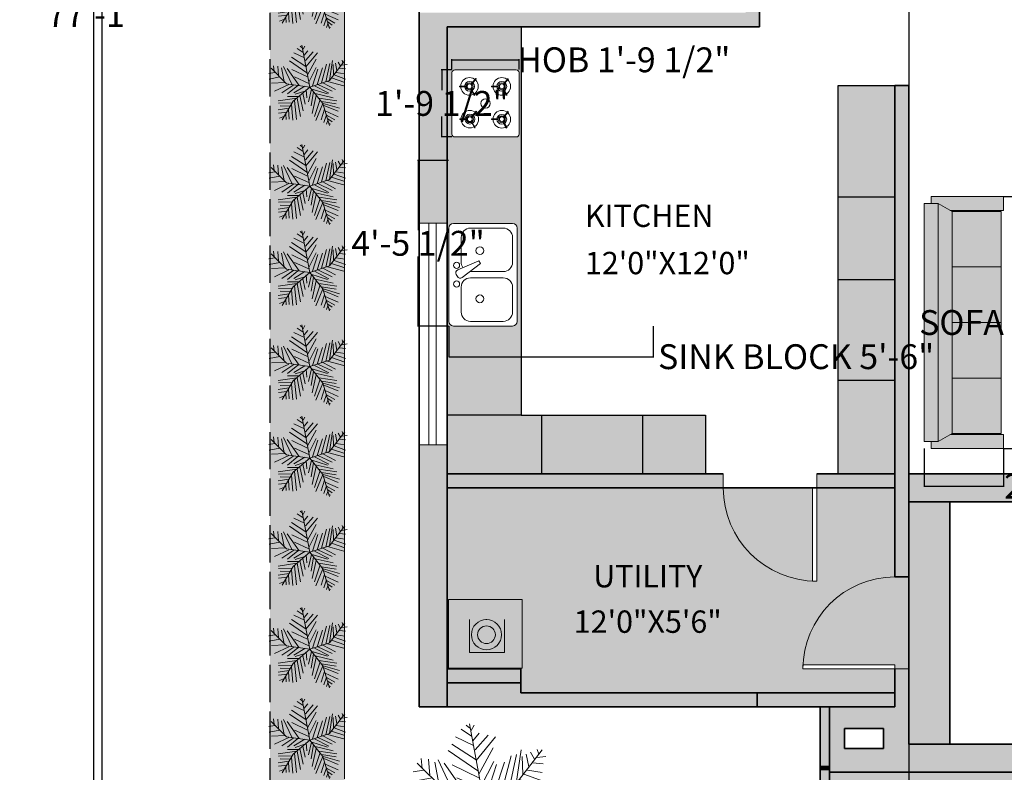
# Model space of a CAD drawing. Units: inches. Extents: x 853 to 1550, y 485 to 1596.
# Tile 2 of 18: x 853 to 1170, y 768 to 1010. Entities that reach past the tile are written whole.
import ezdxf

# ---------------------------------------------------------------- set-up
doc = ezdxf.new("R2010")
doc.units = ezdxf.units.IN
doc.header["$MEASUREMENT"] = 0
doc.linetypes.add('ACAD_ISO02W100', pattern=[15, 12, -3])
for name, color, linetype, lineweight in [('A-ANNO-DIMS', 2, 'Continuous', 18), ('A-AREA-IDEN', 250, 'Continuous', 18), ('A-DOOR', 4, 'Continuous', 18), ('A-EQPM', 8, 'Continuous', 18), ('A-FLOR-CASE', 32, 'Continuous', 25), ('A-FLOR-FIXT', 8, 'Continuous', 18), ('A-WALL-PATT', 250, 'Continuous', 13), ('C-PROP', 8, 'ACAD_ISO02W100', 25), ('furniture', 250, 'Continuous', 18), ('L-PLNT-TREE', 106, 'Continuous', 13), ('lawn', 106, 'Continuous', 18), ('walls', 250, 'Continuous', 35), ('windows', 4, 'Continuous', 18)]:
    doc.layers.add(name, color=color, linetype=linetype, lineweight=lineweight)
for name, color, linetype, lineweight, true_color in [('A-CASE-PATT', 251, 'Continuous', 13, 0x636466), ('A-FIXT-PATT', 9, 'Continuous', 13, 0xc7c8ca), ('A-FLOR-PATT', 254, 'Continuous', 13, 0xfeeab9), ('A-FURN-PATT', 254, 'Continuous', 13, 0xfeeab9), ('L-PLNT-PATT', 85, 'Continuous', 13, 0x58ba48)]:
    doc.layers.add(name, color=color, linetype=linetype, lineweight=lineweight, true_color=true_color)
doc.styles.add('ATT', font='TXT')
doc.styles.get("Standard").update_dxf_attribs({"font": 'arial.ttf'})
doc.dimstyles.get("Standard").update_dxf_attribs({"dimtxt": 8, "dimasz": 0.18, "dimexe": 0.18, "dimexo": 0.0625, "dimgap": 0.09, "dimtad": 0, "dimtih": 1, "dimtoh": 1, "dimzin": 0, "dimdsep": 46, "dimlunit": 3, "dimtxsty": 'Standard', "dimcen": 0.09, "dimadec": 0, "dimazin": 0, "dimtfac": 1, "dimtofl": 0, "dimtmove": 0, "dimatfit": 3, "dimfxl": 1, "dimtolj": 1, "dimtzin": 0, "dimarcsym": 0})

# ---------------------------------------------------------------- blocks, each defined once
blk = doc.blocks.new('15PSNK10')
at = {"color": 0, "linetype": 'ByBlock'}
for p, q in [((20.5, 16.5), (1.5, 16.5)), ((0, 15), (0, -15)), ((7, 15), (17.5, 15)), ((22, -15), (22, 15)), ((4, 4), (4, 12)), ((20.5, 12), (20.5, 4)), ((2.37, -0.1), (2.77, 0.6)), ((10.18, -3.57), (4.27, 0.87)), ((17.5, 1), (7, 1)), ((2.88, -1.54), (9.68, -4.43)), ((7.04, -1), (17.5, -1)), ((4, -12), (4, -4)), ((9.68, -4.43), (10.18, -3.57)), ((20.5, -4), (20.5, -12)), ((17.5, -15), (7, -15)), ((1.5, -16.5), (20.5, -16.5))]:
    blk.add_line(p, q, dxfattribs=at)
for centre, radius in [((10, 7.75), 1.25), ((2.5, 3), 1), ((2.5, -3), 1), ((10, -7.75), 1.25)]:
    blk.add_circle(centre, radius, dxfattribs=at)
for centre, radius, start, end in [((1.5, 15), 1.5, 90, 180), ((20.5, 15), 1.5, 0, 90), ((7, 12), 3, 90, 180), ((17.5, 12), 3, 0, 90), ((7, 4), 3, 180, 270), ((17.5, 4), 3, 270, 0), ((3.63, 0.1), 1, 50.5377, 150), ((3.23, -0.6), 1, 150, 249.4623), ((7, -4), 3, 146.607, 180), ((17.5, -4), 3, 0, 90), ((7, -12), 3, 180, 270), ((17.5, -12), 3, 270, 0), ((1.5, -15), 1.5, 180, 270), ((20.5, -15), 1.5, 270, 0)]:
    blk.add_arc(centre, radius, start, end, dxfattribs=at)
at = {"color": 0, "linetype": 'ByBlock', "style": 'ATT'}
for tag, p, flags in [('ITEM', (0, -26), 3), ('ROOM_NUMBER', (0, -35), 1)]:
    blk.add_attdef(tag, p, '', height=6, dxfattribs=dict(at, flags=flags))
blk = doc.blocks.new('*U10')
for p, q in [((0, 0), (0, -6)), ((40, 0), (40, -6))]:
    blk.add_line(p, q)
blk.add_lwpolyline([(0, 0), (0, 40), (1.75, 40), (1.75, 0)], close=True)
blk.add_arc((0, 0), 40, 0, 90)
blk = doc.blocks.new('FABRIC SOFA 4S')
at = {"layer": 'furniture'}
for p, q in [((0, -51), (0, 51)), ((6, 51), (0, 51)), ((3, 54), (34, 54)), ((3, 51), (3, 54)), ((6, -51), (6, 51)), ((12, 47.63), (6, 51)), ((34, 48), (34, 54)), ((11.14, 48), (34, 48)), ((33, 23.81), (12, 23.81)), ((33, 0), (12, 0)), ((33, -23.81), (12, -23.81)), ((6, -51), (12, -47.63)), ((11.54, -48), (34, -48)), ((34, -48), (34, -54)), ((6, -51), (0, -51)), ((3, -54), (3, -51)), ((3, -54), (34, -54))]:
    blk.add_line(p, q, dxfattribs=at)
blk.add_lwpolyline([(12, -47.63), (12, 47.63), (33, 47.63), (33, -47.63)], close=True, dxfattribs=at)
blk = doc.blocks.new('4bstove')
at = {"layer": 'furniture'}
for p, q in [((1452.73, 1446.21), (1452.73, 1448.61)), ((1452.98, 1446.22), (1452.98, 1448.61)), ((1464.44, 1446.34), (1464.44, 1448.73)), ((1464.69, 1446.34), (1464.69, 1448.73)), ((1451.74, 1444.45), (1449.67, 1443.25)), ((1451.87, 1444.23), (1449.79, 1443.04)), ((1453.75, 1444.08), (1455.58, 1442.54)), ((1453.91, 1444.27), (1455.74, 1442.73)), ((1463.45, 1444.58), (1461.38, 1443.38)), ((1463.57, 1444.36), (1461.5, 1443.17)), ((1465.46, 1444.21), (1467.29, 1442.67)), ((1465.62, 1444.4), (1467.45, 1442.86)), ((1452.69, 1434.81), (1452.69, 1437.2)), ((1452.94, 1434.81), (1452.94, 1437.2)), ((1464.44, 1434.81), (1464.44, 1437.2)), ((1464.69, 1434.81), (1464.69, 1437.2)), ((1451.7, 1433.04), (1449.63, 1431.85)), ((1451.82, 1432.83), (1449.75, 1431.63)), ((1453.87, 1432.86), (1455.7, 1431.33)), ((1463.45, 1433.04), (1461.38, 1431.85)), ((1463.57, 1432.83), (1461.5, 1431.63)), ((1465.62, 1432.86), (1467.45, 1431.33)), ((1453.71, 1432.67), (1455.54, 1431.13)), ((1465.46, 1432.67), (1467.29, 1431.13))]:
    blk.add_line(p, q, dxfattribs=at)
for points in [[(1447.5, 1427.38), (1469.5, 1427.38, 0.414214), (1470.5, 1428.38), (1470.5, 1450.38, 0.414214), (1469.5, 1451.38), (1447.5, 1451.38, 0.414214), (1446.5, 1450.38), (1446.5, 1428.38, 0.414214)], [(1453.75, 1444.97, 1), (1452, 1444.97, 1)], [(1465.46, 1445.1, 1), (1463.71, 1445.1, 1)], [(1453.71, 1433.56, 1), (1451.96, 1433.56, 1)], [(1465.46, 1433.56, 1), (1463.71, 1433.56, 1)]]:
    blk.add_lwpolyline(points, format="xyb", close=True, dxfattribs=at)
for points in [[(1454.12, 1444.97, 1), (1451.62, 1444.97, 1), (1454.12, 1444.97, 1)], [(1465.83, 1445.1, 1), (1463.33, 1445.1, 1), (1465.83, 1445.1, 1)], [(1454.08, 1433.56, 1), (1451.58, 1433.56, 1), (1454.08, 1433.56, 1)], [(1465.83, 1433.56, 1), (1463.33, 1433.56, 1), (1465.83, 1433.56, 1)]]:
    blk.add_lwpolyline(points, format="xyb", dxfattribs=at)
for centre, radius in [((1452.87, 1444.97), 3.14), ((1464.58, 1445.1), 3.14), ((1464.58, 1445.1), 1.75), ((1452.87, 1444.97), 1.75), ((1458.5, 1439.38), 1.67), ((1452.83, 1433.56), 3.14), ((1464.58, 1433.56), 3.14), ((1452.83, 1433.56), 1.75), ((1464.58, 1433.56), 1.75)]:
    blk.add_circle(centre, radius, dxfattribs=at)
for centre, start, end in [((1452.87, 1444.97), 88.2645, 92.2039), ((1464.58, 1445.1), 88.2645, 92.2039), ((1464.58, 1445.1), 208.188, 212.1274), ((1452.87, 1444.97), 208.188, 212.1274), ((1452.87, 1444.97), 318.1018, 322.0412), ((1464.58, 1445.1), 318.1018, 322.0412), ((1452.83, 1433.56), 88.2645, 92.2039), ((1464.58, 1433.56), 88.2645, 92.2039)]:
    blk.add_arc(centre, 3.64, start, end, dxfattribs=at)
blk = doc.blocks.new('stove')
at = {"layer": 'furniture', "xscale": 0.9, "yscale": 0.9, "zscale": 0.9, "rotation": 89.99999999999999}
blk.add_blockref('4bstove', (1295.44, -1312.65), dxfattribs=at)
blk = doc.blocks.new('*U18')
for p, q in [((-10.186, 53.64), (-13.084, 55.962)), ((0, 0), (-10.5, 57)), ((-9.099, 51.782), (-6.563, 55.962)), ((-8.737, 47.138), (-17.069, 52.711)), ((-7.65, 43.423), (-2.578, 49.46)), ((-5.839, 35.992), (4.667, 48.067)), ((-5.114, 28.097), (-24.676, 40.636)), ((-7.288, 39.707), (-21.778, 46.673)), ((-5.114, 27.632), (10.463, 46.673)), ((-3.665, 19.273), (-27.574, 35.527)), ((-2.941, 16.486), (8.652, 37.85)), ((22.055, 7.198), (27.489, 32.277)), ((27, 9), (48, 36)), ((27.127, 9.056), (31.112, 35.992)), ((35.096, 32.741), (37.27, 22.524)), ((38.719, 34.134), (41.979, 28.561)), ((44.153, 36.456), (45.239, 32.741)), ((-31.5, 4.5), (-52.5, 25.5)), ((-48.585, 21.131), (-49.309, 29.026)), ((-43.513, 28.561), (-42.427, 15.558)), ((-38.442, 26.239), (-34.819, 7.663)), ((-35.544, 28.097), (-24.314, 3.947)), ((-14.533, 2.09), (-30.834, 25.31)), ((-24.314, 23.917), (-2.941, 13.7)), ((-1.129, 6.734), (9.014, 26.704)), ((3.942, 1.625), (11.187, 24.381)), ((10.101, 3.483), (17.708, 26.239)), ((16.259, 5.805), (23.142, 31.348)), ((31.836, 30.883), (32.561, 16.486)), ((40.53, 25.775), (48.862, 24.846)), ((43.791, 29.954), (51.036, 30.883)), ((-47.498, 19.737), (-55.83, 18.344)), ((33.285, 16.486), (48.862, 10.913)), ((36.183, 19.737), (48.137, 17.88)), ((-40.615, 13.7), (-55.105, 10.913)), ((-20.691, 13.7), (-1.129, 4.876)), ((0, 0), (27, 9)), ((29.662, 12.307), (48.137, 6.269)), ((-33.37, 6.269), (-52.207, 5.34)), ((-28.299, 3.483), (-47.86, -5.805)), ((-21.416, 3.018), (-38.079, -8.128)), ((0, 0), (-31.5, 4.5)), ((-15.982, 2.09), (-30.11, -9.521)), ((0, 0), (-22.5, -19.5)), ((-6.563, 1.161), (-21.416, -8.128)), ((0, 0), (18, -22.5)), ((6.478, 1.625), (26.04, -8.592)), ((11.187, 3.483), (30.749, -5.805)), ((18.07, 5.805), (35.096, -3.483)), ((24.229, 7.663), (46.688, 1.625)), ((-6.563, -5.805), (-19.967, -9.985)), ((-4.752, -3.483), (-3.665, -14.629)), ((2.493, -3.019), (-1.491, -20.202)), ((1.769, -2.555), (24.229, -9.521)), ((5.029, -6.27), (2.131, -25.775)), ((-17.431, -15.094), (-42.789, -18.809)), ((-15.257, -12.772), (-30.11, -12.772)), ((-17.069, -15.094), (-12.721, -40.172)), ((-13.446, -11.378), (-8.737, -32.741)), ((-9.461, -8.592), (-6.201, -23.453)), ((9.014, -11.378), (3.58, -35.992)), ((7.565, -9.056), (32.198, -14.629)), ((12.274, -15.094), (36.907, -18.809)), ((-24.314, -21.596), (-42.427, -22.06)), ((-22.5, -19.5), (-37.5, -45)), ((-20.691, -18.345), (-17.793, -44.352)), ((14.085, -16.951), (6.478, -40.172)), ((18.07, -22.524), (8.289, -45.745)), ((16.259, -19.738), (36.183, -22.989)), ((18, -22.5), (27, -52.5)), ((18.433, -22.524), (40.53, -29.026)), ((-28.299, -29.026), (-42.789, -31.348)), ((-26.849, -26.24), (-40.253, -25.775)), ((-29.023, -30.884), (-27.936, -43.887)), ((-25.038, -23.918), (-22.865, -45.281)), ((20.244, -30.419), (15.897, -44.816)), ((19.157, -25.311), (38.719, -33.206)), ((-30.834, -34.135), (-42.427, -35.528)), ((-32.646, -36.921), (-31.921, -44.352)), ((22.78, -37.85), (19.519, -48.532)), ((21.331, -32.741), (39.081, -40.636)), ((22.78, -38.314), (34.372, -44.816)), ((-34.457, -39.708), (-40.978, -42.494)), ((24.591, -45.745), (23.142, -50.854)), ((24.591, -43.423), (30.749, -47.603)), ((26.764, -49.925), (28.213, -50.854))]:
    blk.add_line(p, q)
blk = doc.blocks.new('*D23')
at = {"layer": 'A-ANNO-DIMS', "color": 0, "lineweight": -2, "transparency": 16777216}
for p, q in [((879.97, 1474.13), (879.75, 1474.13)), ((879.93, 1473.95), (879.93, 1049.11)), ((879.93, 615.92), (879.93, 1040.76)), ((879.97, 615.74), (879.75, 615.74))]:
    blk.add_line(p, q, dxfattribs=at)
at = {"layer": 'A-ANNO-DIMS', "color": 0, "transparency": 16777216}
for points in [[(879.9, 1473.95), (879.96, 1473.95), (879.93, 1474.13)], [(879.9, 615.92), (879.96, 615.92), (879.93, 615.74)]]:
    blk.add_solid(points, dxfattribs=at)
at = {"layer": 'Defpoints', "color": 0, "transparency": 16777216}
for p in [(880.03, 1474.13), (879.93, 615.74), (880.03, 615.74)]:
    blk.add_point(p, dxfattribs=at)
at = {"layer": 'A-ANNO-DIMS', "color": 0, "transparency": 16777216, "insert": (879.93, 1044.94), "char_height": 8, "attachment_point": 5}
blk.add_mtext("\\A1;60'", dxfattribs=at)
blk = doc.blocks.new('WIN-71IN')
for p, q in [((0, 9), (0, 0)), ((71.43, 9), (0, 9)), ((0, 9), (0, 5.92)), ((71.43, 0), (71.43, 9)), ((0, 5.92), (71.43, 5.92)), ((71.43, 3.59), (0, 3.59)), ((71.43, 5.92), (71.43, 3.59)), ((0, 0), (71.43, 0))]:
    blk.add_line(p, q)
blk = doc.blocks.new('*D49')
at = {"layer": 'A-ANNO-DIMS', "color": 0, "lineweight": -2, "transparency": 16777216}
for p, q in [((1169.96, 952.92), (1182.24, 952.92)), ((1182.06, 952.74), (1182.06, 916.61)), ((1182.06, 872.02), (1182.06, 908.15)), ((1169.96, 871.84), (1182.24, 871.84))]:
    blk.add_line(p, q, dxfattribs=at)
at = {"layer": 'A-ANNO-DIMS', "color": 0, "transparency": 16777216}
for points in [[(1182.03, 952.74), (1182.09, 952.74), (1182.06, 952.92)], [(1182.03, 872.02), (1182.09, 872.02), (1182.06, 871.84)]]:
    blk.add_solid(points, dxfattribs=at)
at = {"layer": 'Defpoints', "color": 0, "transparency": 16777216}
for p in [(1169.9, 952.92), (1182.06, 952.92), (1169.9, 871.84)]:
    blk.add_point(p, dxfattribs=at)
at = {"layer": 'A-ANNO-DIMS', "color": 0, "transparency": 16777216, "insert": (1182.06, 912.38), "char_height": 8, "attachment_point": 5}
blk.add_mtext('\\A1;SOFA 6\'-9" TYP.', dxfattribs=at)
blk = doc.blocks.new('*D50')
at = {"layer": 'A-ANNO-DIMS', "color": 0, "lineweight": -2, "transparency": 16777216}
for p, q in [((1144.37, 871.78), (1144.37, 859.5)), ((1169.9, 871.78), (1169.9, 859.5)), ((1144.55, 859.68), (1169.72, 859.68)), ((1169.9, 859.68), (1170.08, 859.68))]:
    blk.add_line(p, q, dxfattribs=at)
at = {"layer": 'A-ANNO-DIMS', "color": 0, "transparency": 16777216}
for points in [[(1144.55, 859.71), (1144.55, 859.65), (1144.37, 859.68)], [(1169.72, 859.71), (1169.72, 859.65), (1169.9, 859.68)]]:
    blk.add_solid(points, dxfattribs=at)
at = {"layer": 'Defpoints', "color": 0, "transparency": 16777216}
for p in [(1144.37, 871.84), (1169.9, 871.84), (1169.9, 859.68)]:
    blk.add_point(p, dxfattribs=at)
at = {"layer": 'A-ANNO-DIMS', "color": 0, "transparency": 16777216, "insert": (1203.94, 859.68), "char_height": 8, "attachment_point": 5}
blk.add_mtext('\\A1;2\'-1 1/2" TYP.', dxfattribs=at)
blk = doc.blocks.new('*D63')
at = {"layer": 'A-ANNO-DIMS', "color": 0, "lineweight": -2, "transparency": 16777216}
for p, q in [((991.44, 911.19), (991.44, 901.2)), ((1057.24, 911.19), (1057.24, 901.2)), ((991.62, 901.38), (1057.06, 901.38)), ((1057.24, 901.38), (1057.42, 901.38))]:
    blk.add_line(p, q, dxfattribs=at)
at = {"layer": 'A-ANNO-DIMS', "color": 0, "transparency": 16777216}
for points in [[(991.62, 901.41), (991.62, 901.35), (991.44, 901.38)], [(1057.06, 901.41), (1057.06, 901.35), (1057.24, 901.38)]]:
    blk.add_solid(points, dxfattribs=at)
at = {"layer": 'Defpoints', "color": 0, "transparency": 16777216}
for p in [(991.44, 911.25), (1057.24, 911.25), (1057.24, 901.38)]:
    blk.add_point(p, dxfattribs=at)
at = {"layer": 'A-ANNO-DIMS', "color": 0, "transparency": 16777216, "insert": (1103.22, 901.38), "char_height": 8, "attachment_point": 5}
blk.add_mtext('\\A1;SINK BLOCK 5\'-6"', dxfattribs=at)
blk = doc.blocks.new('*D64')
at = {"layer": 'A-ANNO-DIMS', "color": 0, "lineweight": -2, "transparency": 16777216}
for p, q in [((991.38, 964.51), (981.39, 964.51)), ((981.57, 964.33), (981.57, 942.11)), ((981.57, 911.43), (981.57, 933.66)), ((991.38, 911.25), (981.39, 911.25))]:
    blk.add_line(p, q, dxfattribs=at)
at = {"layer": 'A-ANNO-DIMS', "color": 0, "transparency": 16777216}
for points in [[(981.54, 964.33), (981.6, 964.33), (981.57, 964.51)], [(981.54, 911.43), (981.6, 911.43), (981.57, 911.25)]]:
    blk.add_solid(points, dxfattribs=at)
at = {"layer": 'Defpoints', "color": 0, "transparency": 16777216}
for p in [(991.44, 964.51), (981.57, 911.25), (991.44, 911.25)]:
    blk.add_point(p, dxfattribs=at)
at = {"layer": 'A-ANNO-DIMS', "color": 0, "transparency": 16777216, "insert": (981.57, 937.88), "char_height": 8, "attachment_point": 5}
blk.add_mtext('\\A1;4\'-5 1/2"', dxfattribs=at)
blk = doc.blocks.new('*D65')
at = {"layer": 'A-ANNO-DIMS', "color": 0, "lineweight": -2, "transparency": 16777216}
for p, q in [((992.47, 993.79), (992.47, 997.14)), ((992.65, 996.96), (1013.89, 996.96)), ((1014.07, 993.79), (1014.07, 997.14)), ((1014.07, 996.96), (1014.25, 996.96))]:
    blk.add_line(p, q, dxfattribs=at)
at = {"layer": 'A-ANNO-DIMS', "color": 0, "transparency": 16777216}
for points in [[(992.65, 996.99), (992.65, 996.93), (992.47, 996.96)], [(1013.89, 996.99), (1013.89, 996.93), (1014.07, 996.96)]]:
    blk.add_solid(points, dxfattribs=at)
at = {"layer": 'Defpoints', "color": 0, "transparency": 16777216}
for p in [(1014.07, 996.96), (992.47, 993.72), (1014.07, 993.72)]:
    blk.add_point(p, dxfattribs=at)
at = {"layer": 'A-ANNO-DIMS', "color": 0, "transparency": 16777216, "insert": (1047.74, 996.96), "char_height": 8, "attachment_point": 5}
blk.add_mtext('\\A1;HOB 1\'-9 1/2"', dxfattribs=at)
blk = doc.blocks.new('*D66')
at = {"layer": 'A-ANNO-DIMS', "color": 0, "lineweight": -2, "transparency": 16777216}
for p, q in [((992.41, 993.72), (989.05, 993.72)), ((989.23, 993.54), (989.23, 987.15)), ((989.23, 972.3), (989.23, 978.7)), ((992.41, 972.12), (989.05, 972.12))]:
    blk.add_line(p, q, dxfattribs=at)
at = {"layer": 'A-ANNO-DIMS', "color": 0, "transparency": 16777216}
for points in [[(989.2, 993.54), (989.26, 993.54), (989.23, 993.72)], [(989.2, 972.3), (989.26, 972.3), (989.23, 972.12)]]:
    blk.add_solid(points, dxfattribs=at)
at = {"layer": 'Defpoints', "color": 0, "transparency": 16777216}
for p in [(989.23, 993.72), (992.47, 993.72), (992.47, 972.12)]:
    blk.add_point(p, dxfattribs=at)
at = {"layer": 'A-ANNO-DIMS', "color": 0, "transparency": 16777216, "insert": (989.23, 982.92), "char_height": 8, "attachment_point": 5}
blk.add_mtext('\\A1;1\'-9 1/2"', dxfattribs=at)
blk = doc.blocks.new('*D70')
at = {"layer": 'A-ANNO-DIMS', "color": 0, "lineweight": -2, "transparency": 16777216}
for p, q in [((981.87, 1426.13), (877.09, 1426.13)), ((877.27, 1425.95), (877.27, 1067.22)), ((877.27, 700.05), (877.27, 1058.77)), ((1110.88, 699.87), (877.09, 699.87))]:
    blk.add_line(p, q, dxfattribs=at)
at = {"layer": 'A-ANNO-DIMS', "color": 0, "transparency": 16777216}
for points in [[(877.24, 1425.95), (877.3, 1425.95), (877.27, 1426.13)], [(877.24, 700.05), (877.3, 700.05), (877.27, 699.87)]]:
    blk.add_solid(points, dxfattribs=at)
at = {"layer": 'Defpoints', "color": 0, "transparency": 16777216}
for p in [(981.94, 1426.13), (877.27, 699.87), (1110.94, 699.87)]:
    blk.add_point(p, dxfattribs=at)
at = {"layer": 'A-ANNO-DIMS', "color": 0, "transparency": 16777216, "insert": (877.27, 1063), "char_height": 8, "attachment_point": 5}
blk.add_mtext('\\A1;60\'-6 1/2"', dxfattribs=at)
blk = doc.blocks.new('*D71')
at = {"layer": 'A-ANNO-DIMS', "color": 0, "lineweight": -2, "transparency": 16777216}
for p, q in [((933.87, 1474.13), (877.09, 1474.13)), ((877.27, 1473.95), (877.27, 1015.66)), ((877.27, 549.16), (877.27, 1007.45)), ((933.87, 548.98), (877.09, 548.98))]:
    blk.add_line(p, q, dxfattribs=at)
at = {"layer": 'A-ANNO-DIMS', "color": 0, "transparency": 16777216}
for points in [[(877.24, 1473.95), (877.3, 1473.95), (877.27, 1474.13)], [(877.24, 549.16), (877.3, 549.16), (877.27, 548.98)]]:
    blk.add_solid(points, dxfattribs=at)
at = {"layer": 'Defpoints', "color": 0, "transparency": 16777216}
for p in [(877.27, 1474.13), (933.94, 1474.13), (933.94, 548.98)]:
    blk.add_point(p, dxfattribs=at)
at = {"layer": 'A-ANNO-DIMS', "color": 0, "transparency": 16777216, "insert": (877.27, 1011.55), "char_height": 8, "attachment_point": 5}
blk.add_mtext('\\A1;77\'-1"', dxfattribs=at)
blk = doc.blocks.new('*D72')
at = {"layer": 'A-ANNO-DIMS', "color": 0, "lineweight": -2, "transparency": 16777216}
for p, q in [((1139.44, 1321.07), (1139.44, 497.1)), ((1199.44, 1321.07), (1199.44, 497.1)), ((1139.62, 497.28), (1158.71, 497.28)), ((1199.26, 497.28), (1180.16, 497.28))]:
    blk.add_line(p, q, dxfattribs=at)
at = {"layer": 'A-ANNO-DIMS', "color": 0, "transparency": 16777216}
for points in [[(1139.62, 497.31), (1139.62, 497.25), (1139.44, 497.28)], [(1199.26, 497.31), (1199.26, 497.25), (1199.44, 497.28)]]:
    blk.add_solid(points, dxfattribs=at)
at = {"layer": 'Defpoints', "color": 0, "transparency": 16777216}
for p in [(1139.44, 1321.13), (1199.44, 1321.13), (1199.44, 497.28)]:
    blk.add_point(p, dxfattribs=at)
at = {"layer": 'A-ANNO-DIMS', "color": 0, "transparency": 16777216, "insert": (1169.44, 497.28), "char_height": 8, "attachment_point": 5}
blk.add_mtext('\\A1;5\'-0"', dxfattribs=at)

msp = doc.modelspace()

# ---------------------------------------------------------------- hatches: boundary and pattern name
at = {"layer": 'A-CASE-PATT'}
h = msp.add_hatch(color=256, dxfattribs=at)
h.dxf.hatch_style = 1
h.paths.add_polyline_path([(1014.791, 1007.629), (990.937, 1007.629), (990.937, 882.565), (1014.791, 882.565)])
h.paths.add_polyline_path([(993.371, 972.124, -0.4142136), (992.471, 973.024), (992.471, 992.824, -0.4142136), (993.371, 993.724), (1013.171, 993.724, -0.4142136), (1014.071, 992.824), (1014.071, 973.024, -0.4142136), (1013.171, 972.124)], flags=16)
h.paths.add_polyline_path([(999.785, 974.974), (999.56, 975.364, -0.5505708), (995.418, 977.733), (994.968, 977.733, -0.0171907), (994.967, 977.958), (995.417, 977.958, -0.6105283), (999.962, 980.094), (1000.252, 980.439, -0.0171906), (1000.425, 980.295), (1000.135, 979.95, -0.2116406), (1001.062, 977.859, -0.2564461), (999.754, 975.477), (999.979, 975.087, -0.0171907)], flags=0)
h.paths.add_polyline_path([(996.664, 977.859, -1), (999.814, 977.859, -1)], flags=0)
h.paths.add_polyline_path([(1005.686, 977.694), (1005.235, 977.694, -0.0171907), (1005.234, 977.919), (1005.685, 977.919, -0.9825922), (1011.329, 977.82, -0.9779445)], flags=0)
h.paths.add_polyline_path([(998.239, 976.734, -1), (998.239, 978.984, -1)], flags=0)
h.paths.add_polyline_path([(998.239, 977.071, -1), (998.239, 978.646, -1)], flags=0)
h.paths.add_polyline_path([(1006.931, 977.82, -1), (1010.081, 977.82, -1)], flags=0)
h.paths.add_polyline_path([(1008.506, 976.695, -1), (1008.506, 978.945, -1)], flags=0)
h.paths.add_polyline_path([(1008.506, 978.608, -1), (1008.506, 977.033, -1)], flags=0)
h.paths.add_polyline_path([(1001.768, 982.924, -1), (1004.775, 982.924, -1)], flags=0)
h.paths.add_polyline_path([(1011.963, 944.284, -0.4142136), (1013.464, 942.783), (1013.464, 912.755, -0.4142136), (1011.963, 911.254), (992.945, 911.254, -0.4142136), (991.444, 912.755), (991.444, 942.783, -0.4142136), (992.945, 944.284)], flags=16)
h.paths.add_polyline_path([(1001.131, 932.206), (1001.632, 931.339), (995.718, 926.897, -0.4631975), (994.215, 927.169), (993.812, 927.867, -0.4369407), (994.246, 929.271)], flags=0)
h.paths.add_polyline_path([(999.67, 985.51), (999.445, 985.9, -0.5505708), (995.304, 988.269), (994.853, 988.269, -0.0171907), (994.852, 988.494), (995.303, 988.494, -0.6105283), (999.848, 990.63), (1000.137, 990.975, -0.0171906), (1000.31, 990.831), (1000.02, 990.486, -0.2116406), (1000.947, 988.395, -0.2564461), (999.639, 986.013), (999.865, 985.623, -0.0171907)], flags=0)
h.paths.add_polyline_path([(1005.686, 988.269), (1005.235, 988.269, -0.0171907), (1005.234, 988.494), (1005.685, 988.494, -0.9825922), (1011.329, 988.395, -0.9779445)], flags=0)
h.paths.add_polyline_path([(996.549, 988.395, -1), (999.699, 988.395, -1)], flags=0)
h.paths.add_polyline_path([(1006.931, 988.395, -1), (1010.081, 988.395, -1)], flags=0)
h.paths.add_polyline_path([(1008.506, 987.27, -1), (1008.506, 989.52, -1)], flags=0)
h.paths.add_polyline_path([(998.124, 987.27, -1), (998.124, 989.52, -1)], flags=0)
h.paths.add_polyline_path([(998.124, 987.607, -1), (998.124, 989.182, -1)], flags=0)
h.paths.add_polyline_path([(1008.506, 989.182, -1), (1008.506, 987.607, -1)], flags=0)
h.paths.add_polyline_path([(1002.704, 935.526, -1), (1000.202, 935.526, -1)], flags=0)
h.paths.add_polyline_path([(994.947, 930.772, -1), (992.945, 930.772, -1)], flags=0)
h.paths.add_polyline_path([(1008.96, 926.768, -0.4142136), (1011.963, 923.765), (1011.963, 915.758, -0.4142136), (1008.96, 912.755), (998.451, 912.755, -0.4142136), (995.448, 915.758), (995.448, 923.765, -0.4142136), (998.451, 926.768)], flags=0)
h.paths.add_polyline_path([(994.947, 924.766, -1), (992.945, 924.766, -1)], flags=0)
h.paths.add_polyline_path([(1002.704, 920.012, -1), (1000.202, 920.012, -1)], flags=0)
h.paths.add_polyline_path([(1074.071, 882.565), (1053.829, 882.565), (1053.829, 863.629), (1074.071, 863.629)])
h.paths.add_polyline_path([(1134.937, 988.732), (1116.786, 988.732), (1116.786, 952.856), (1134.937, 952.856)])
h = msp.add_hatch(color=256, dxfattribs=at)
h.dxf.hatch_style = 1
h.paths.add_polyline_path([(1021.322, 882.565), (1014.791, 882.565), (990.937, 882.565), (990.937, 872.981), (990.937, 863.629), (1021.322, 863.629)])
h.paths.add_polyline_path([(1053.829, 882.565), (1021.322, 882.565), (1021.322, 863.629), (1053.829, 863.629)])
h.paths.add_polyline_path([(1134.937, 952.856), (1116.786, 952.856), (1116.786, 926.18), (1134.937, 926.18)])
h.paths.add_polyline_path([(1134.937, 926.18), (1116.786, 926.18), (1116.786, 893.867), (1134.937, 893.867)])
h.paths.add_polyline_path([(1134.937, 893.867), (1116.786, 893.867), (1116.786, 863.629), (1134.937, 863.629)])
at = {"layer": 'A-FIXT-PATT'}
h = msp.add_hatch(color=256, dxfattribs=at)
h.dxf.hatch_style = 1
h.paths.add_polyline_path([(1003.276, 820.953), (993.274, 820.953), (993.274, 801.121), (1014.49, 801.121), (1014.49, 820.953), (1003.882, 820.953, -0.4044775), (1012.667, 811.87, -1), (994.491, 811.87, -0.4044775)])
h = msp.add_hatch(color=256, dxfattribs=at)
h.dxf.hatch_style = 1
h.paths.add_polyline_path([(1003.882, 820.953), (1003.276, 820.953, 0.4044775), (994.491, 811.87, 1), (1012.667, 811.87, 0.4044775)])
h.paths.add_polyline_path([(1008.934, 811.87, -1), (998.224, 811.87, -1)], flags=16)
h = msp.add_hatch(color=256, dxfattribs=at)
h.dxf.hatch_style = 1
h.paths.add_polyline_path([(1000.72, 811.87, 1), (1006.437, 811.87, 1)])
at = {"layer": 'A-FLOR-PATT'}
h = msp.add_hatch(color=256, dxfattribs=at)
h.dxf.hatch_style = 1
h.paths.add_polyline_path([(1079.778, 859.129), (990.937, 859.129), (990.937, 800.886), (1014.605, 800.886), (1014.605, 796.386), (1014.605, 793.129), (1134.937, 793.129), (1134.937, 800.892), (1105.418, 800.892), (1105.418, 802.186), (1105.447, 802.186, -0.4008371), (1134.937, 830.473), (1134.937, 859.129), (1109.834, 859.129), (1109.834, 829.107), (1108.519, 829.107), (1108.519, 829.136, -0.4011291)])
h.paths.add_polyline_path([(1139.437, 830.473), (1135, 830.473, 0.4014527), (1105.447, 802.186), (1135, 802.186), (1135, 800.892), (1139.437, 800.892)])
h.paths.add_polyline_path([(1108.519, 859.129), (1079.778, 859.129, 0.4011291), (1108.519, 829.136)], flags=17)
h = msp.add_hatch(color=256, dxfattribs=at)
h.dxf.hatch_style = 1
h.paths.add_polyline_path([(1152.624, 854.629), (1139.437, 854.629), (1139.437, 776.629), (1152.624, 776.629)])
h = msp.add_hatch(color=256, dxfattribs=at)
h.dxf.hatch_style = 1
h.paths.add_polyline_path([(1090.727, 793.129), (1014.605, 793.129), (1014.605, 796.386), (990.937, 796.386), (990.937, 788.629), (1090.727, 788.629)])
h = msp.add_hatch(color=256, dxfattribs=at)
h.dxf.hatch_style = 1
h.paths.add_polyline_path([(1113.94, 788.629), (1110.94, 788.629), (1110.94, 769.463), (1113.94, 769.463)])
h.paths.add_polyline_path([(1113.94, 768.501), (1110.94, 768.501), (1110.94, 707.356), (1113.94, 707.356)])
h.paths.add_polyline_path([(1276.896, 702.868), (1118.963, 702.868), (1118.963, 699.868), (1276.896, 699.868)])
h.paths.add_polyline_path([(1284.919, 770.496), (1261.179, 770.496), (1261.179, 767.496), (1281.919, 767.496), (1281.919, 707.356), (1284.919, 707.356)])
h = msp.add_hatch(color=256, dxfattribs=at)
h.dxf.hatch_style = 1
h.paths.add_polyline_path([(1113.94, 769.463), (1110.94, 769.463), (1110.94, 768.501), (1113.94, 768.501)])
h = msp.add_hatch(color=256, dxfattribs=at)
h.dxf.hatch_style = 1
h.paths.add_polyline_path([(1281.919, 767.496), (1261.179, 767.496), (1113.94, 767.629), (1113.94, 707.356), (1118.963, 707.356), (1118.963, 702.868), (1276.896, 702.868), (1276.896, 707.356), (1281.919, 707.356)])
at = {"layer": 'A-FURN-PATT'}
h = msp.add_hatch(color=256, dxfattribs=at)
h.dxf.hatch_style = 1
h.paths.add_polyline_path([(1148.879, 950.672), (1146.626, 950.672), (1146.626, 952.924), (1169.9, 952.924), (1169.9, 948.42), (1152.883, 948.42)], flags=16)
h.paths.add_polyline_path([(1148.879, 874.094), (1148.879, 950.672), (1153.383, 948.138), (1153.383, 876.628)], flags=16)
h.paths.add_polyline_path([(1144.374, 874.094), (1144.374, 950.672), (1148.879, 950.672), (1148.879, 874.094)], flags=17)
h.paths.add_polyline_path([(1153.383, 876.628), (1153.383, 948.138), (1152.883, 948.42), (1169.9, 948.42), (1169.9, 952.924), (1146.626, 952.924), (1146.626, 950.672), (1144.374, 950.672), (1144.374, 874.094), (1146.626, 874.094), (1146.626, 871.842), (1169.9, 871.842), (1169.9, 876.346), (1152.883, 876.346)])
h = msp.add_hatch(color=256, dxfattribs=at)
h.dxf.hatch_style = 1
h.paths.add_polyline_path([(1152.883, 948.42), (1148.879, 950.672), (1146.626, 950.672), (1146.626, 952.924), (1169.9, 952.924), (1169.9, 948.42)])
h.paths.add_polyline_path([(1148.879, 874.094), (1148.879, 950.672), (1153.383, 948.138), (1153.383, 876.628)])
h.paths.add_polyline_path([(1144.374, 874.094), (1144.374, 950.672), (1148.879, 950.672), (1148.879, 874.094)])
h = msp.add_hatch(color=256, dxfattribs=at)
h.dxf.hatch_style = 1
h.paths.add_polyline_path([(1153.383, 948.138), (1169.149, 948.138), (1169.149, 930.261), (1153.383, 930.261)])
h.paths.add_polyline_path([(1153.383, 930.261), (1169.149, 930.261), (1169.149, 912.383), (1153.383, 912.383)])
h.paths.add_polyline_path([(1153.383, 912.383), (1169.149, 912.383), (1169.149, 894.506), (1153.383, 894.506)])
h.paths.add_polyline_path([(1153.383, 894.506), (1169.149, 894.506), (1169.149, 876.628), (1153.383, 876.628)])
at = {"layer": 'A-WALL-PATT'}
h = msp.add_hatch(color=256, dxfattribs=at)
h.dxf.hatch_style = 1
h.paths.add_polyline_path([(1139.437, 988.732), (1134.937, 988.732), (1134.937, 830.473), (1139.437, 830.473)])
h.paths.add_polyline_path([(1413.937, 1052.227), (1404.937, 1052.227), (1404.937, 1036.129), (1308.937, 1036.129), (1308.937, 1045.033), (1304.437, 1045.033), (1304.437, 1030.033), (1308.937, 1030.033), (1308.937, 1031.629), (1404.937, 1031.629), (1404.937, 863.629), (1365.241, 863.629), (1365.241, 854.629), (1413.937, 854.629)])
h.paths.add_polyline_path([(1413.937, 1133.918), (1404.937, 1133.918), (1404.937, 1100.629), (1304.437, 1100.629), (1304.437, 1078.26), (1308.937, 1078.26), (1308.937, 1096.129), (1404.937, 1096.129), (1404.937, 1084.233), (1407.946, 1084.233), (1413.937, 1084.233)])
h.paths.add_polyline_path([(1268.437, 1417.129), (1288.974, 1417.129), (1288.974, 1426.129), (1244.597, 1426.129), (1244.597, 1417.129), (1263.937, 1417.129), (1263.937, 1321.129), (1260.34, 1321.129), (1260.34, 1316.629), (1263.937, 1316.629), (1263.937, 1283.505), (1268.437, 1283.505)])
h.paths.add_polyline_path([(1413.937, 1426.129), (1360.402, 1426.129), (1360.402, 1417.129), (1404.937, 1417.129), (1404.937, 1249.129), (1268.437, 1249.129), (1268.437, 1254.041), (1268.357, 1254.041), (1263.937, 1254.041), (1263.937, 1244.629), (1404.937, 1244.629), (1404.937, 1228.163), (1413.937, 1228.163)])
h.paths.add_polyline_path([(1215.842, 1426.129), (1184.201, 1426.129), (1184.201, 1417.129), (1199.437, 1417.129), (1199.437, 1321.129), (1172.101, 1321.129), (1172.101, 1316.629), (1229.433, 1316.629), (1229.433, 1321.129), (1203.937, 1321.129), (1203.937, 1417.129), (1215.842, 1417.129)])
h.paths.add_polyline_path([(1139.437, 1417.129), (1155.446, 1417.129), (1155.446, 1426.129), (1091.831, 1426.129), (1091.831, 1417.129), (1134.937, 1417.129), (1134.937, 1289.22), (1139.437, 1289.22), (1139.437, 1316.629), (1143.553, 1316.629), (1143.553, 1321.129), (1139.437, 1321.129)])
h.paths.add_polyline_path([(1139.437, 1255.161), (1134.937, 1255.161), (1134.937, 1249.129), (990.937, 1249.129), (990.937, 1417.129), (1020.402, 1417.129), (1020.402, 1426.129), (981.937, 1426.129), (981.937, 1205.535), (984.477, 1205.535), (990.937, 1205.535), (990.937, 1244.629), (1134.937, 1244.629), (1134.937, 1237.775), (1139.437, 1237.775)])
h = msp.add_hatch(color=256, dxfattribs=at)
h.dxf.hatch_style = 1
h.paths.add_polyline_path([(990.937, 1111.29), (981.937, 1111.29), (981.937, 1044.136), (984.946, 1044.136), (990.937, 1044.136), (990.937, 1072.129), (1045.609, 1072.129, -0.0272078), (1045.453, 1074.983), (1045.453, 1076.629), (990.937, 1076.629)], flags=17)
h.paths.add_polyline_path([(1091.437, 1072.129), (1139.437, 1072.129), (1139.437, 1206.521), (1134.937, 1206.521), (1134.937, 1076.629), (1071.734, 1076.629), (1071.734, 1074.983), (1071.734, 1072.129), (1086.937, 1072.129), (1086.937, 1012.129), (990.937, 1012.129), (981.937, 1012.129), (981.937, 944.409), (990.937, 944.409), (990.937, 1007.629), (1091.437, 1007.629)])
h.paths.add_polyline_path([(990.937, 872.981), (981.937, 872.981), (981.937, 788.629), (990.937, 788.629)])
h.paths.add_polyline_path([(1014.605, 800.886), (990.937, 800.886), (990.937, 796.386), (1014.605, 796.386)])
h.paths.add_polyline_path([(1134.937, 793.129), (1090.727, 793.129), (1090.727, 788.629), (1134.937, 788.629)])
h.paths.add_polyline_path([(1139.437, 800.892), (1134.937, 800.892), (1134.937, 788.629), (1113.94, 788.629), (1113.94, 767.629), (1139.437, 767.629), (1191.938, 767.629), (1191.938, 772.657), (1191.938, 776.629), (1139.437, 776.629)])
h.paths.add_polyline_path([(1131.331, 781.621), (1131.331, 775.236), (1118.809, 775.236), (1118.809, 781.621)], flags=16)
h.paths.add_polyline_path([(1131.331, 781.621), (1118.809, 781.621), (1118.809, 775.236), (1131.331, 775.236)], flags=0)
h.paths.add_polyline_path([(1118.963, 707.356), (1110.94, 707.356), (1110.94, 699.868), (1118.963, 699.868)])
h.paths.add_polyline_path([(1284.919, 707.356), (1276.896, 707.356), (1276.896, 699.868), (1284.919, 699.868)])
h.paths.add_polyline_path([(1293.812, 863.629), (1268.437, 863.629), (1268.437, 984.936), (1308.937, 984.936), (1308.937, 996.627), (1304.437, 996.627), (1304.437, 989.436), (1263.937, 989.436), (1263.937, 863.629), (1215.364, 863.629), (1215.364, 854.629), (1252.179, 854.629), (1252.179, 776.629), (1225.216, 776.629, -0.0297134), (1225.453, 772.657), (1225.453, 767.629), (1261.179, 767.629), (1261.179, 854.629), (1293.812, 854.629)])
h.paths.add_polyline_path([(1176.151, 863.629), (1139.437, 863.629), (1139.437, 854.629), (1176.151, 854.629)])
h.paths.add_polyline_path([(1134.937, 863.629), (1109.834, 863.629), (1109.834, 859.129), (1134.937, 859.129)])
h.paths.add_polyline_path([(1148.879, 950.672), (1144.374, 950.672), (1144.374, 874.094), (1148.879, 874.094)])
h.paths.add_polyline_path([(1079.778, 863.629), (990.937, 863.629), (990.937, 859.129), (1079.778, 859.129)])
at = {"layer": 'L-PLNT-PATT'}
h = msp.add_hatch(color=256, dxfattribs=at)
h.dxf.hatch_style = 1
h.paths.add_polyline_path([(1461.937, 1474.129), (933.937, 1474.129), (933.937, 730.129), (933.937, 622.891), (941.686, 622.891), (941.686, 604.895), (957.937, 604.895), (957.937, 1450.129), (1437.937, 1450.129), (1437.937, 604.895), (1454.646, 604.895), (1454.646, 622.891), (1461.937, 622.891), (1461.937, 734.988)])

# ---------------------------------------------------------------- linework, layer by layer
at = {"layer": 'A-EQPM'}
for p, q in [((991.95, 823.154), (991.387, 823.154)), ((991.387, 823.154), (991.387, 821.364)), ((991.387, 801.136), (991.387, 821.364)), ((991.95, 823.154), (1015.055, 823.154)), ((1015.055, 817.178), (1015.055, 823.154)), ((998.078, 806.132), (998.078, 816.718)), ((1003.417, 816.718), (1003.741, 816.718)), ((1009.403, 816.718), (1009.403, 806.132)), ((1015.055, 817.178), (1015.055, 801.136)), ((1009.403, 806.132), (998.078, 806.132)), ((1015.055, 801.136), (991.387, 801.136))]:
    msp.add_line(p, q, dxfattribs=at)
for radius in [4.851, 2.858]:
    msp.add_circle((1003.579, 811.87), radius, dxfattribs=at)
at = {"layer": 'A-FLOR-CASE'}
for p, q in [((1014.791, 1007.629), (1014.791, 882.565)), ((1116.786, 863.629), (1116.786, 988.732)), ((1116.786, 988.732), (1134.937, 988.732)), ((1116.786, 952.856), (1134.937, 952.856)), ((1116.786, 926.18), (1134.937, 926.18)), ((1116.786, 893.867), (1134.937, 893.867)), ((1014.791, 882.565), (990.937, 882.565)), ((1014.791, 882.565), (1074.071, 882.565)), ((1021.322, 882.565), (1021.322, 863.629)), ((1053.829, 882.565), (1053.829, 863.629)), ((1074.071, 882.565), (1074.071, 863.629))]:
    msp.add_line(p, q, dxfattribs=at)
at = {"layer": 'C-PROP'}
msp.add_line((933.937, 730.129), (933.937, 1474.129), dxfattribs=at)
at = {"layer": 'lawn'}
msp.add_line((957.937, 765.455), (957.937, 1450.129), dxfattribs=at)
at = {"layer": 'walls'}
for p, q in [((981.937, 788.629), (981.937, 1426.129)), ((1091.437, 1007.629), (1091.437, 1072.129)), ((990.937, 788.629), (990.937, 1007.629)), ((990.937, 1007.629), (1091.437, 1007.629)), ((1134.937, 988.732), (1139.437, 988.732)), ((1134.937, 830.473), (1134.937, 988.732)), ((1139.437, 776.629), (1139.437, 988.732)), ((990.937, 863.629), (1079.778, 863.629)), ((1109.834, 863.629), (1134.937, 863.629)), ((1139.437, 863.629), (1176.151, 863.629)), ((990.937, 859.129), (1134.937, 859.129)), ((1139.437, 854.629), (1176.151, 854.629)), ((1152.624, 776.629), (1152.624, 854.629)), ((1135, 830.473), (1139.437, 830.473)), ((1014.605, 800.886), (990.937, 800.886)), ((1014.605, 796.386), (1014.605, 800.886)), ((1134.937, 788.629), (1134.937, 800.892)), ((990.937, 796.386), (1014.605, 796.386)), ((1014.605, 796.386), (1014.605, 793.129)), ((1014.605, 793.129), (1134.937, 793.129)), ((1014.605, 793.129), (1090.727, 793.129)), ((1090.727, 793.129), (1014.605, 793.129)), ((1090.727, 793.129), (1014.605, 793.129)), ((1090.727, 793.129), (1090.727, 788.629)), ((981.937, 788.629), (1134.937, 788.629)), ((1110.94, 788.629), (1110.94, 699.868)), ((1113.94, 767.629), (1113.94, 788.629)), ((1113.94, 788.629), (1113.94, 707.356)), ((1118.809, 781.621), (1131.331, 781.621)), ((1118.809, 775.236), (1118.809, 781.621)), ((1131.331, 781.621), (1131.331, 775.236)), ((1139.437, 776.629), (1191.938, 776.629)), ((1131.331, 775.236), (1118.809, 775.236)), ((1110.94, 769.463), (1113.94, 769.463)), ((1113.94, 768.501), (1110.94, 768.501)), ((1113.94, 769.463), (1113.94, 768.501)), ((1113.94, 767.629), (1261.179, 767.629)), ((1139.437, 767.629), (1113.94, 767.629))]:
    msp.add_line(p, q, dxfattribs=at)

# ---------------------------------------------------------------- block references
at = {"layer": 'A-DOOR'}
for p, xscale, yscale, zscale, rotation in [((1109.834, 859.163), 0.7513956278525376, 0.7513956278525376, 0.7513956278525376, 180), ((1135, 800.892), 0.7395414901997985, 0.7395414901997985, 0.7395414901997985, 90)]:
    msp.add_blockref('*U10', p, dxfattribs=dict(at, xscale=xscale, yscale=yscale, zscale=zscale, rotation=rotation))
at = {"layer": 'A-EQPM'}
msp.add_blockref('stove', (1003.271, 982.924), dxfattribs=at)
at = {"layer": 'A-FLOR-FIXT', "xscale": -1.000923628257447, "yscale": 1.000923628257447, "zscale": 1.000923628257447, "rotation": 180}
msp.add_blockref('15PSNK10', (991.444, 927.769), dxfattribs=at)
at = {"layer": 'furniture', "xscale": 0.7507637528364199, "yscale": 0.7507637528364199, "zscale": 0.7507637528364199}
msp.add_blockref('FABRIC SOFA 4S', (1144.374, 912.383), dxfattribs=at)
at = {"layer": 'L-PLNT-TREE'}
for p, xscale, yscale, zscale in [((946.691, 1019.378), 0.2357951711934384, 0.2357951711934384, 0.2357951711934384), ((946.691, 988.203), 0.2357951711934384, 0.2357951711934384, 0.2357951711934384), ((946.691, 956.281), 0.2357951711934384, 0.2357951711934384, 0.2357951711934384), ((946.691, 928.508), 0.2357951711934384, 0.2357951711934384, 0.2357951711934384), ((946.691, 898.182), 0.2357951711934384, 0.2357951711934384, 0.2357951711934384), ((946.691, 868.747), 0.2357951711934384, 0.2357951711934384, 0.2357951711934384), ((946.691, 838.407), 0.2357951711934384, 0.2357951711934384, 0.2357951711934384), ((946.691, 807.172), 0.2357951711934384, 0.2357951711934384, 0.2357951711934384), ((946.691, 777.957), 0.2357951711934384, 0.2357951711934384, 0.2357951711934384), ((1002.291, 760.365), 0.3996992985476591, 0.3996992985476591, 0.3996992985476591)]:
    msp.add_blockref('*U18', p, dxfattribs=dict(at, xscale=xscale, yscale=yscale, zscale=zscale))
at = {"layer": 'windows', "rotation": 89.99999999999976}
msp.add_blockref('WIN-71IN', (990.937, 872.981), dxfattribs=at)

# ---------------------------------------------------------------- texts
at = {"layer": 'A-AREA-IDEN'}
for s, height, p in [('KITCHEN', 7.1944, (1035.249, 943.147)), ('12\'0"X12\'0"', 7.19435, (1035.249, 927.928)), ('UTILITY', 7.1944, (1037.917, 827.115)), ('12\'0"X5\'6"', 7.1944, (1031.661, 812.472))]:
    msp.add_text(s, height=height, dxfattribs=at).set_placement(p)

# ---------------------------------------------------------------- dimensions: what is measured, and where the dimension line sits
at = {"layer": 'A-ANNO-DIMS'}
for base, p1, p2, angle, picture, middle in [((877.2718, 1474.1293), (933.9371, 548.9788), (933.9371, 1474.1293), 90, '*D71', (877.2718, 1011.5541)), ((877.272, 699.868), (981.937, 1426.129), (1110.94, 699.868), 90, '*D70', (877.272, 1062.999)), ((989.231, 993.724), (992.471, 972.124), (992.471, 993.724), 90, '*D66', (989.231, 982.924)), ((981.574, 911.254), (991.444, 964.515), (991.444, 911.254), 270, '*D64', (981.574, 937.884))]:
    dim = msp.add_linear_dim(base=base, p1=p1, p2=p2, angle=angle, dimstyle='Standard', override={"dimdec": 1, "dimlfac": 1, "dimrnd": 0, "dimzin": 1, "dimdsep": 46, "dimlunit": 4, "dimfrac": 2}, dxfattribs=at)
    dim.commit()
    dim.dimension.update_dxf_attribs({"geometry": picture, "text_midpoint": middle})
for base, p1, p2, text, override, picture, middle in [((879.933, 615.743), (880.035, 1474.129), (880.035, 615.743), "60'", {"dimclrd": 0, "dimclre": 0, "dimclrt": 0}, '*D23', (879.933, 1044.936)), ((1182.062, 952.924), (1169.9, 871.842), (1169.9, 952.924), 'SOFA <> TYP.', {"dimdec": 1, "dimlfac": 1, "dimrnd": 0, "dimzin": 1, "dimdsep": 46, "dimlunit": 4, "dimfrac": 2}, '*D49', (1182.062, 912.383))]:
    dim = msp.add_linear_dim(base=base, p1=p1, p2=p2, angle=90, text=text, dimstyle='Standard', override=override, dxfattribs=at)
    dim.commit()
    dim.dimension.update_dxf_attribs({"geometry": picture, "text_midpoint": middle})
dim = msp.add_linear_dim(base=(1199.437, 497.279), p1=(1139.437, 1321.129), p2=(1199.437, 1321.129), dimstyle='Standard', override={"dimdec": 1, "dimlfac": 1, "dimrnd": 0, "dimzin": 1, "dimdsep": 46, "dimlunit": 4, "dimfrac": 2}, dxfattribs=at)
dim.commit()
dim.dimension.update_dxf_attribs({"geometry": '*D72', "text_midpoint": (1169.437, 497.279)})
for base, p1, p2, text, picture, middle in [((1014.071, 996.964), (992.471, 993.724), (1014.071, 993.724), 'HOB <>', '*D65', (1047.741, 996.964)), ((1057.244, 901.384), (991.444, 911.254), (1057.244, 911.254), 'SINK BLOCK <>', '*D63', (1103.219, 901.384)), ((1169.9, 859.68), (1144.374, 871.842), (1169.9, 871.842), '<> TYP.', '*D50', (1203.941, 859.68))]:
    dim = msp.add_linear_dim(base=base, p1=p1, p2=p2, text=text, dimstyle='Standard', override={"dimdec": 1, "dimlfac": 1, "dimrnd": 0, "dimzin": 1, "dimdsep": 46, "dimlunit": 4, "dimfrac": 2}, dxfattribs=at)
    dim.commit()
    dim.dimension.update_dxf_attribs({"geometry": picture, "text_midpoint": middle})

doc.saveas('drawing.dxf')
